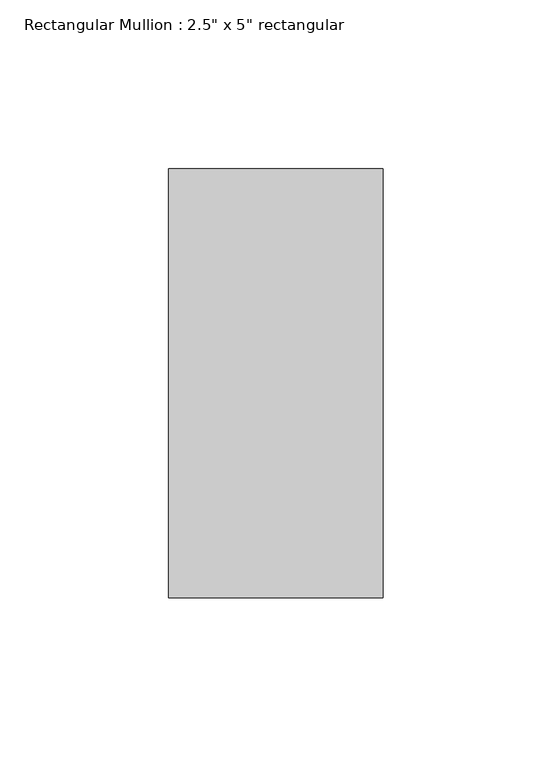
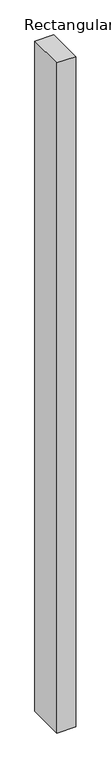
"""IFC4 building model written with IfcOpenShell, lengths in millimetres: member geometry."""

from ifc_helpers import new_model, si_unit, frame, origin, place, context, project, spatial, polyline, outline, extrude, source, transform, mapped, element, save


def member_d1af338a(model_context):
    return source(origin(), model_context, "Body", "SweptSolid", [
        extrude(outline(polyline([(0.0, 63.5), (0.0, -63.5), (-63.5, -63.5), (-63.5, 63.5), (0.0, 63.5)])), frame((0.0, 0.0, -2370.6666667), z_axis=(0.0, 0.0, 1.0), x_axis=(1.0, 0.0, 0.0)), (0.0, 0.0, 1.0), 2370.6666667),
    ])


if __name__ == "__main__":
    model = new_model("IFC4")
    model_context = context("Model", 3, world=origin())
    ifc_project = project(units=[si_unit("LENGTHUNIT", "METRE", prefix="MILLI")], contexts=[model_context])
    site = spatial("IfcSite", under=ifc_project)
    building = spatial("IfcBuilding", under=site)
    placement = place(None, origin())
    member_shape = member_d1af338a(model_context)
    element("IfcMember", 1, ObjectType="Rectangular Mullion : 2.5\" x 5\" rectangular", at=placement, inside=building, context=model_context, shape_type="MappedRepresentation", body=[
        mapped(member_shape, transform((0.0, 0.0, 0.0), x_axis=(1.0, 0.0, 0.0), y_axis=(0.0, 1.0, 0.0), z_axis=(0.0, 0.0, 1.0))),
    ])
    save(model, "model.ifc")

# Revit data of these elements
# Type "Rectangular Mullion : 2.5\" x 5\" rectangular"
#   built-in parameter 1007304 = 0.416667 (stored number, unit not read)
#   built-in parameter 1007301 = 0.104167 (stored number, unit not read)
#   built-in parameter 1007300 = 0.104167 (stored number, unit not read)
# Element 1 (IfcMember, "Rectangular Mullion : 2.5\" x 5\" rectangular")
#   Materials on its faces: "Aluminum"
# Materials
#   "Aluminum": class "Metal", colour RGB 247 247 247, transparency 0, Description = "Aluminum 6061", Cost = 0
